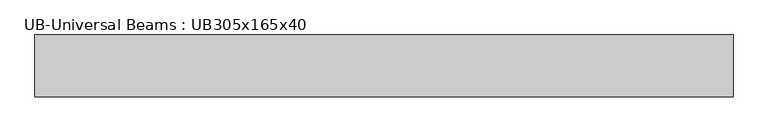
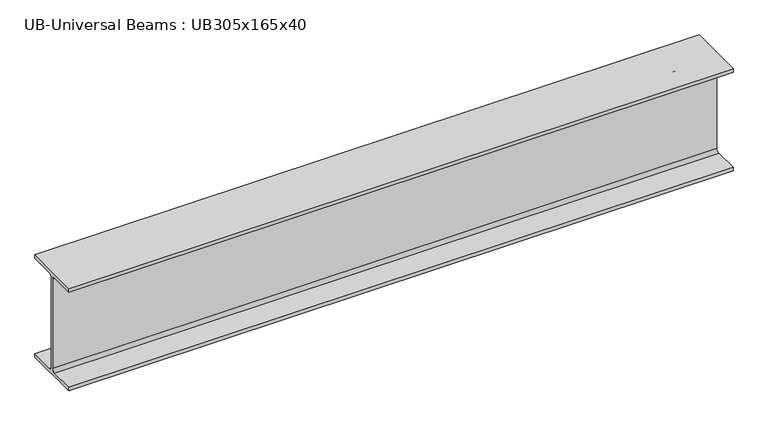
"""IFC4 building model written with IfcOpenShell, lengths in millimetres: beam geometry, UB-Universal Beams : UB305x165x40."""

from ifc_helpers import new_model, si_unit, point, frame, frame_2d, origin, place, context, project, spatial, polyline, circle_curve, trimmed, segment, composite_curve, outline, extrude, source, transform, mapped, element, save


def ub_universal_beams_ub305x165x40_28de461c(model_context):
    return source(origin(), model_context, "Body", "SweptSolid", [
        extrude(outline(composite_curve([segment(polyline([(82.5, -141.5), (82.5, -151.7), (-82.5, -151.7), (-82.5, -141.5), (-11.9, -141.5)]), True, "CONTINUOUS"), segment(trimmed(circle_curve(frame_2d((-11.9, -132.6)), 8.9), [point((-11.9, -141.5))], [point((-3.0, -132.6))], True, "CARTESIAN"), True, "CONTINUOUS"), segment(polyline([(-3.0, -132.6), (-3.0, 132.6)]), True, "CONTINUOUS"), segment(trimmed(circle_curve(frame_2d((-11.9, 132.6)), 8.9), [point((-3.0, 132.6))], [point((-11.9, 141.5))], True, "CARTESIAN"), True, "CONTINUOUS"), segment(polyline([(-11.9, 141.5), (-82.5, 141.5), (-82.5, 151.7), (82.5, 151.7), (82.5, 141.5), (11.9, 141.5)]), True, "CONTINUOUS"), segment(trimmed(circle_curve(frame_2d((11.9, 132.6)), 8.9), [point((11.9, 141.5))], [point((3.0, 132.6))], True, "CARTESIAN"), True, "CONTINUOUS"), segment(polyline([(3.0, 132.6), (3.0, -132.6)]), True, "CONTINUOUS"), segment(trimmed(circle_curve(frame_2d((11.9, -132.6)), 8.9), [point((3.0, -132.6))], [point((11.9, -141.5))], True, "CARTESIAN"), True, "CONTINUOUS"), segment(polyline([(11.9, -141.5), (82.5, -141.5)]), True, "CONTINUOUS")], self_intersect=False)), frame((-825.65, 0.0, 0.0), z_axis=(1.0, 0.0, 0.0), x_axis=(0.0, 1.0, 0.0)), (0.0, 0.0, 1.0), 1863.5),
    ])


if __name__ == "__main__":
    model = new_model("IFC4")
    model_context = context("Model", 3, world=origin())
    ifc_project = project(units=[si_unit("LENGTHUNIT", "METRE", prefix="MILLI")], contexts=[model_context])
    site = spatial("IfcSite", under=ifc_project)
    building = spatial("IfcBuilding", under=site)
    placement = place(None, origin())
    ub_universal_beams_ub305x165x40_shape = ub_universal_beams_ub305x165x40_28de461c(model_context)
    element("IfcBeam", 1, ObjectType="UB-Universal Beams : UB305x165x40", at=placement, inside=building, context=model_context, shape_type="MappedRepresentation", body=[
        mapped(ub_universal_beams_ub305x165x40_shape, transform((0.0, 0.0, 0.0), x_axis=(1.0, 0.0, 0.0), y_axis=(0.0, 1.0, 0.0), z_axis=(0.0, 0.0, 1.0))),
    ])
    save(model, "model.ifc")

# Revit data of these elements
# Type "UB-Universal Beams : UB305x165x40"
#   Section Name Key = "UB305X165X40"
#   Width = 16.5 cm
#   Web Thickness = 0.6 cm
#   Web Fillet = 0.89 cm
#   Warping Constant = 164000.0 cm⁶
#   Torsional Moment of Inertia = 14.70 cm⁴
#   Section Area = 51.3 cm²
#   Plastic Modulus weak axis = 142.0 cm³
#   Plastic Modulus strong axis = 623.0 cm³
#   Nominal Weight = 40.2999 kgf/m
#   Moment of Inertia weak axis = 764.00 cm⁴
#   Moment of Inertia strong axis = 8503.00 cm⁴
#   Height = 30.34 cm
#   Flange Thickness = 1.02 cm
#   Elastic Modulus weak axis = 92.6 cm³
#   Elastic Modulus strong axis = 560.0 cm³
#   Centroid Vertical = 15.17 cm
#   Centroid Horizontal = 8.25 cm
#   Bolt Spacing = 9.0 cm
#   Length [instance default] = 1500 mm
#   Structural Material [instance default] = Metal - Steel 43-275
#   Type Comments = ""
#   Assembly Code = ""
# Element 1 (IfcBeam, "UB-Universal Beams : UB305x165x40")
#   Materials on its faces: "Metal - Steel 43-275"
# Materials
#   "Metal - Steel 43-275": class "Metal", colour RGB 247 247 247, transparency 0, Cost = 0
